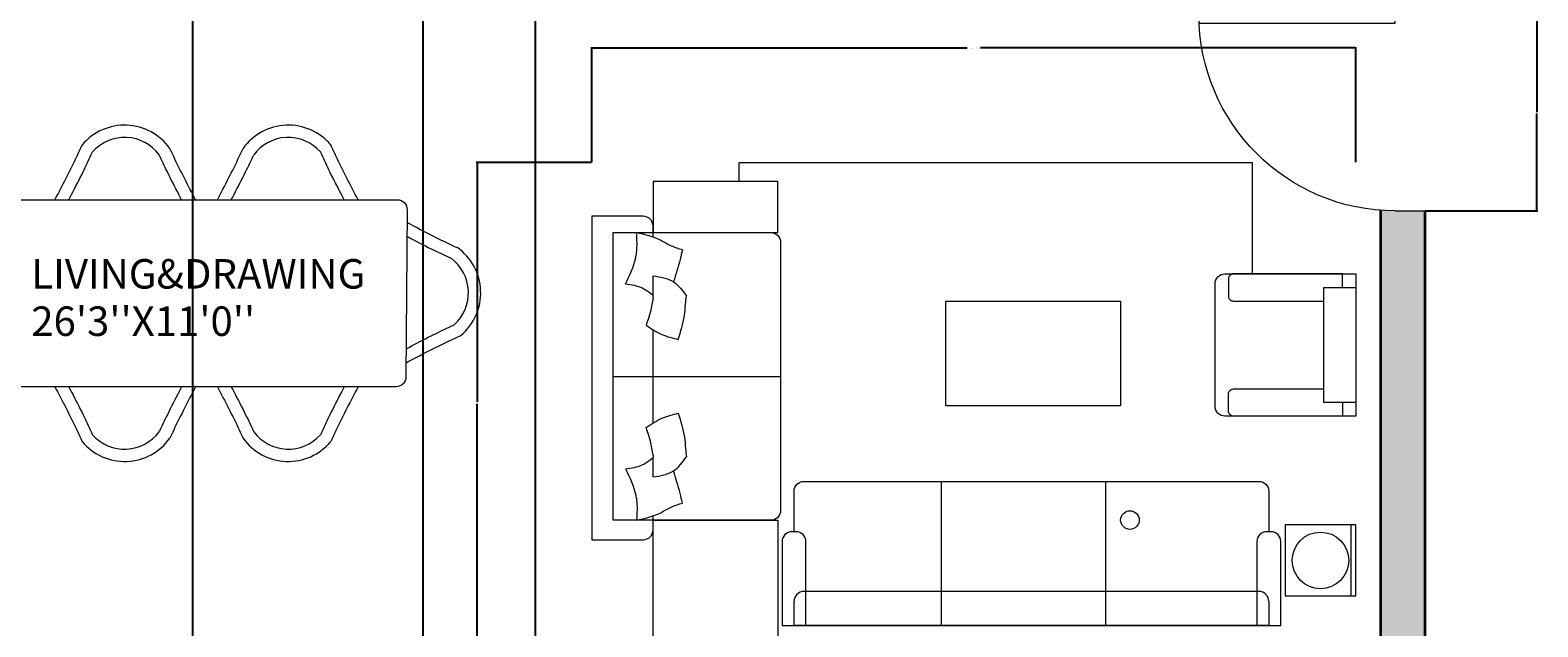
# Model space of a CAD drawing. Units: inches. Extents: x 1789 to 2841, y 3180 to 3702.
# Tile 5 of 14: x 2041 to 2348, y 3388 to 3510. Entities that reach past the tile are written whole.
import ezdxf

# ---------------------------------------------------------------- set-up
doc = ezdxf.new("R2010")
doc.units = ezdxf.units.IN
doc.header["$MEASUREMENT"] = 0
for name, color, linetype, lineweight in [('A-ANNO-DIMS', 2, 'Continuous', 18), ('A-AREA-IDEN', 7, 'Continuous', 18), ('A-WALL', 40, 'Continuous', 35), ('A-WALL-PATT', 252, 'Continuous', 13), ('DORS', 70, 'Continuous', 18), ('FURNITURE', 34, 'Continuous', 18)]:
    doc.layers.add(name, color=color, linetype=linetype, lineweight=lineweight)
doc.styles.get("Standard").update_dxf_attribs({"font": 'arial.ttf'})
doc.dimstyles.get("Standard").update_dxf_attribs({"dimtxt": 0.18, "dimasz": 0.18, "dimexe": 0.18, "dimexo": 0.0625, "dimgap": 0.09, "dimtad": 0, "dimtih": 1, "dimtoh": 1, "dimdec": 0, "dimzin": 0, "dimdsep": 46, "dimlunit": 3, "dimtxsty": 'Standard', "dimcen": 0.09, "dimadec": 0, "dimazin": 0, "dimtfac": 1, "dimtdec": 0, "dimtofl": 0, "dimtmove": 0, "dimatfit": 3, "dimfxl": 1, "dimtolj": 1, "dimtzin": 0, "dimarcsym": 0})

# ---------------------------------------------------------------- blocks, each defined once
blk = doc.blocks.new('*U26')
for p, q in [((0, 0), (0, -6)), ((40, 0), (40, -6))]:
    blk.add_line(p, q)
blk.add_lwpolyline([(0, 0), (0, 40), (1.75, 40), (1.75, 0)], close=True)
blk.add_arc((0, 0), 40, 0, 90)
blk = doc.blocks.new('SOFA')
for p, q in [((2185.57, 3479.13), (2185.57, 3482.99)), ((2185.57, 3482.99), (2290.09, 3482.99)), ((2290.09, 3482.99), (2290.09, 3460.33)), ((2159.93, 3439.46), (2194.03, 3439.46)), ((2226.79, 3388.76), (2226.79, 3418.07)), ((2260.29, 3388.76), (2260.29, 3418.07)), ((2310.14, 3409.22), (2310.14, 3394.77))]:
    blk.add_line(p, q)
for points in [[(2168.05, 3468.75), (2193.44, 3468.75), (2193.44, 3479.13), (2168.05, 3479.13)], [(2227.7, 3454.8), (2263.24, 3454.8), (2263.24, 3433.45), (2227.7, 3433.45)], [(2304.69, 3457.56), (2311.21, 3457.56), (2311.21, 3434.14), (2304.69, 3434.14)], [(2168.05, 3410.16), (2193.44, 3410.16), (2193.44, 3385.14), (2168.05, 3385.14)], [(2296.77, 3394.77), (2311.21, 3394.77), (2311.21, 3409.22), (2296.77, 3409.22)]]:
    blk.add_lwpolyline(points, close=True)
for points in [[(2168.05, 3467.86), (2168.05, 3470.06, 0.414214), (2166.05, 3472.06), (2155.57, 3472.06), (2155.57, 3406.2), (2166.05, 3406.2, 0.414214), (2168.05, 3408.2), (2168.05, 3411.06)], [(2308.49, 3457.56), (2308.49, 3460.33), (2286.26, 3460.33, 0.414214), (2285.26, 3459.33), (2285.26, 3455.79, 0.414214), (2286.26, 3454.79), (2304.69, 3454.79)], [(2308.49, 3434.14), (2308.49, 3431.37), (2286.26, 3431.37, -0.414214), (2285.26, 3432.37), (2285.26, 3435.9, -0.414214), (2286.26, 3436.9), (2304.69, 3436.9)], [(2196.77, 3407.83), (2196.77, 3416.07, -0.414214), (2198.77, 3418.07), (2291.47, 3418.07, -0.414214), (2293.47, 3416.07), (2293.47, 3407.83)], [(2293.47, 3393.66, 0.414214), (2291.47, 3395.66), (2198.77, 3395.66, 0.414214), (2196.77, 3393.66)]]:
    blk.add_lwpolyline(points, format="xyb")
for points in [[(2159.93, 3468.75), (2192.03, 3468.75, -0.414214), (2194.03, 3466.75), (2194.03, 3412.16, -0.414214), (2192.03, 3410.16), (2159.93, 3410.16)], [(2284.53, 3460.33), (2311.21, 3460.33), (2311.21, 3431.37), (2284.53, 3431.37, -0.414214), (2282.53, 3433.37), (2282.53, 3458.33, -0.414214)], [(2197.2, 3407.83), (2196.33, 3407.83, 0.414214), (2194.33, 3405.83), (2194.33, 3388.76), (2199.2, 3388.76), (2199.2, 3405.83, 0.414214)], [(2293.91, 3407.83), (2293.04, 3407.83, 0.414214), (2291.04, 3405.83), (2291.04, 3388.76), (2295.91, 3388.76), (2295.91, 3405.83, 0.414214)]]:
    blk.add_lwpolyline(points, format="xyb", close=True)
for points in [[(2168.05, 3455.52), (2168.05, 3459.94)], [(2168.05, 3429.95), (2168.05, 3448.97)], [(2168.05, 3423.4), (2168.05, 3422.93)], [(2168.05, 3418.98), (2168.05, 3422.93)], [(2293.47, 3393.66), (2293.47, 3388.76), (2196.77, 3388.76), (2196.77, 3393.66)], [(2196.77, 3388.76), (2293.47, 3388.76)]]:
    blk.add_lwpolyline(points)
for centre, radius in [((2265.18, 3410.2), 1.89), ((2303.99, 3401.99), 5.76)]:
    blk.add_circle(centre, radius)
for points, knots in [([(2162.46, 3458.3), (2163.29, 3460.04), (2164.26, 3462.07), (2164.89, 3465.65), (2164.78, 3467.36), (2164.69, 3468.75)], [0, 0, 0, 0, 5.733795, 6.696566, 10.854822, 10.854822, 10.854822, 10.854822]), ([(2164.69, 3468.75), (2166.38, 3468.37), (2168.87, 3467.8), (2171.7, 3465.95), (2173.26, 3465.49), (2174.05, 3465.25)], [0, 0, 0, 0, 5.14676, 7.56322, 10.027291, 10.027291, 10.027291, 10.027291]), ([(2174.05, 3465.25), (2173.89, 3464.58), (2173.37, 3462.38), (2172.69, 3460.22), (2172.22, 3458.71)], [0, 0, 0, 0, 2.055182, 6.796603, 6.796603, 6.796603, 6.796603]), ([(2162.46, 3458.3), (2163.64, 3458.13), (2165.71, 3457.83), (2167.35, 3456.54), (2168.05, 3455.99)], [0, 0, 0, 0, 3.512009, 6.140853, 6.140853, 6.140853, 6.140853]), ([(2168.05, 3459.94), (2169.55, 3459.7), (2172.38, 3459.25), (2174.06, 3456.94), (2174.85, 3455.84)], [0, 0, 0, 0, 4.35123, 8.24052, 8.24052, 8.24052, 8.24052]), ([(2173.18, 3446.97), (2173.68, 3448.57), (2174.42, 3450.93), (2174.65, 3453.95), (2174.79, 3455.29), (2174.85, 3455.84)], [0, 0, 0, 0, 5.016146, 7.373936, 9.056838, 9.056838, 9.056838, 9.056838]), ([(2166.66, 3449.86), (2167.7, 3449.17), (2169.71, 3447.85), (2172.05, 3447.25), (2173.18, 3446.97)], [0, 0, 0, 0, 3.710874, 7.178588, 7.178588, 7.178588, 7.178588]), ([(2166.66, 3429.05), (2167.7, 3429.74), (2169.71, 3431.07), (2172.05, 3431.66), (2173.18, 3431.95)], [0, 0, 0, 0, 3.710874, 7.178588, 7.178588, 7.178588, 7.178588]), ([(2173.18, 3431.95), (2173.68, 3430.35), (2174.42, 3427.99), (2174.65, 3424.97), (2174.79, 3423.63), (2174.85, 3423.07)], [0, 0, 0, 0, 5.016146, 7.373936, 9.056838, 9.056838, 9.056838, 9.056838]), ([(2162.46, 3420.62), (2163.64, 3420.79), (2165.71, 3421.09), (2167.35, 3422.37), (2168.05, 3422.93)], [0, 0, 0, 0, 3.512009, 6.140853, 6.140853, 6.140853, 6.140853]), ([(2168.05, 3418.98), (2169.55, 3419.22), (2172.38, 3419.66), (2174.06, 3421.98), (2174.85, 3423.07)], [0, 0, 0, 0, 4.35123, 8.24052, 8.24052, 8.24052, 8.24052]), ([(2162.46, 3420.62), (2163.29, 3418.88), (2164.26, 3416.85), (2164.89, 3413.27), (2164.78, 3411.56), (2164.69, 3410.16)], [0, 0, 0, 0, 5.733795, 6.696566, 10.854822, 10.854822, 10.854822, 10.854822]), ([(2174.05, 3413.67), (2173.89, 3414.33), (2173.37, 3416.54), (2172.69, 3418.7), (2172.22, 3420.21)], [0, 0, 0, 0, 2.055182, 6.796603, 6.796603, 6.796603, 6.796603]), ([(2164.69, 3410.16), (2166.38, 3410.55), (2168.87, 3411.12), (2171.7, 3412.96), (2173.26, 3413.43), (2174.05, 3413.67)], [0, 0, 0, 0, 5.14676, 7.56322, 10.027291, 10.027291, 10.027291, 10.027291])]:
    blk.add_open_spline(points, degree=3, knots=knots)
for points in [[(2168.05, 3455.52), (2167.85, 3453.6), (2167.25, 3451.73), (2166.66, 3449.86)], [(2168.05, 3423.4), (2167.85, 3425.31), (2167.25, 3427.18), (2166.66, 3429.05)]]:
    blk.add_open_spline(points, degree=3)
blk = doc.blocks.new('DINI')
blk.add_lwpolyline([(2038.22, 3475.42), (2115.97, 3475.42, -0.414214), (2117.97, 3473.42), (2117.72, 3439.35, -0.414214), (2115.72, 3437.35), (2037.97, 3437.35, -0.414214), (2035.97, 3439.35), (2036.22, 3473.42, -0.414214)], format="xyb", close=True)
for centre, radius, start, end in [((2060.43, 3479.31), 11.31, 35.4017, 140.0736), ((2093.76, 3479.31), 11.31, 39.9264, 144.5983), ((2060.43, 3479.31), 8.8, 36.8657, 137.9611), ((2093.76, 3479.31), 8.8, 42.0389, 143.1343), ((2032.05, 3456.46), 11.31, 125.4017, 230.0736), ((2121.64, 3456.46), 11.31, 309.9264, 54.5983), ((2032.05, 3456.46), 8.8, 126.8657, 227.9611), ((2121.64, 3456.46), 8.8, 312.0389, 53.1343), ((2060.43, 3433.45), 8.8, 222.0389, 323.1343), ((2093.76, 3433.45), 8.8, 216.8657, 317.9611), ((2060.43, 3433.45), 11.31, 219.9264, 324.5983), ((2093.76, 3433.45), 11.31, 215.4017, 320.0736)]:
    blk.add_arc(centre, radius, start, end)
for points, knots in [([(2046.22, 3475.42), (2047.75, 3478.33), (2049.68, 3482.01), (2051.4, 3485.79), (2051.76, 3486.58)], [0, 0, 0, 0, 7.856931, 9.915256, 9.915256, 9.915256, 9.915256]), ([(2074.88, 3475.42), (2073.35, 3478.33), (2071.54, 3481.78), (2069.91, 3485.32), (2069.66, 3485.87)], [0, 0, 0, 0, 7.856931, 9.297576, 9.297576, 9.297576, 9.297576]), ([(2079.31, 3475.42), (2080.85, 3478.33), (2082.66, 3481.78), (2084.29, 3485.32), (2084.54, 3485.87)], [0, 0, 0, 0, 7.856931, 9.297576, 9.297576, 9.297576, 9.297576]), ([(2107.98, 3475.42), (2106.45, 3478.33), (2104.51, 3482.01), (2102.79, 3485.79), (2102.44, 3486.58)], [0, 0, 0, 0, 7.856931, 9.915256, 9.915256, 9.915256, 9.915256]), ([(2049.05, 3475.42), (2049.25, 3475.79), (2049.44, 3476.15), (2050.42, 3478.03), (2051.21, 3479.56), (2052.54, 3482.27), (2053.1, 3483.45), (2053.72, 3484.82), (2053.81, 3485.01), (2053.9, 3485.21)], [1.048693, 1.048693, 1.048693, 1.048693, 2.029233, 2.029233, 6.0877, 6.0877, 9.118148, 9.118148, 9.624349, 9.624349, 9.624349, 9.624349]), ([(2072.04, 3475.42), (2071.85, 3475.78), (2071.66, 3476.15), (2070.68, 3478.03), (2069.89, 3479.55), (2068.56, 3482.26), (2068.01, 3483.43), (2067.48, 3484.59)], [1.048889, 1.048889, 1.048889, 1.048889, 2.02655, 2.02655, 6.079649, 6.079649, 9.095857, 9.095857, 9.095857, 9.095857]), ([(2082.15, 3475.42), (2082.34, 3475.78), (2082.53, 3476.15), (2083.51, 3478.03), (2084.3, 3479.55), (2085.63, 3482.26), (2086.19, 3483.43), (2086.72, 3484.59)], [1.048889, 1.048889, 1.048889, 1.048889, 2.02655, 2.02655, 6.079649, 6.079649, 9.095857, 9.095857, 9.095857, 9.095857]), ([(2105.14, 3475.42), (2104.95, 3475.79), (2104.76, 3476.15), (2103.78, 3478.03), (2102.99, 3479.56), (2101.65, 3482.27), (2101.1, 3483.45), (2100.47, 3484.82), (2100.38, 3485.01), (2100.3, 3485.21)], [1.048693, 1.048693, 1.048693, 1.048693, 2.029233, 2.029233, 6.0877, 6.0877, 9.118148, 9.118148, 9.624349, 9.624349, 9.624349, 9.624349]), ([(2036.2, 3471.04), (2036.05, 3470.96), (2035.89, 3470.88), (2035.74, 3470.8), (2035.74, 3470.8), (2035.74, 3470.8), (2035.74, 3470.8), (2032.89, 3469.3), (2029.51, 3467.53), (2026.05, 3465.93), (2025.5, 3465.68)], [-0.229823, -0.229823, -0.229823, -0.229823, 0.189373, 0.189373, 0.189373, 0.189712, 0.189712, 0.189712, 7.856931, 9.297576, 9.297576, 9.297576, 9.297576]), ([(2117.95, 3470.8), (2120.8, 3469.3), (2124.18, 3467.53), (2127.64, 3465.93), (2128.19, 3465.68)], [0.189712, 0.189712, 0.189712, 0.189712, 7.856931, 9.297576, 9.297576, 9.297576, 9.297576]), ([(2036.18, 3468.19), (2036.04, 3468.12), (2035.9, 3468.04), (2035.76, 3467.97), (2035.76, 3467.97), (2035.76, 3467.97), (2035.76, 3467.97), (2035.46, 3467.81), (2035.16, 3467.65), (2033.34, 3466.71), (2031.81, 3465.92), (2029.11, 3464.59), (2027.94, 3464.04), (2026.77, 3463.5)], [0.838882, 0.838882, 0.838882, 0.838882, 1.215073, 1.215073, 1.215073, 1.219193, 1.219193, 1.219193, 2.02655, 2.02655, 6.079649, 6.079649, 9.095857, 9.095857, 9.095857, 9.095857]), ([(2117.93, 3467.97), (2118.23, 3467.81), (2118.53, 3467.65), (2120.35, 3466.71), (2121.88, 3465.92), (2124.58, 3464.59), (2125.75, 3464.04), (2126.92, 3463.5)], [1.219193, 1.219193, 1.219193, 1.219193, 2.02655, 2.02655, 6.079649, 6.079649, 9.095857, 9.095857, 9.095857, 9.095857]), ([(2035.95, 3445.08), (2035.58, 3445.27), (2035.22, 3445.46), (2033.34, 3446.45), (2031.81, 3447.23), (2029.1, 3448.57), (2027.92, 3449.12), (2026.55, 3449.75), (2026.36, 3449.84), (2026.16, 3449.93)], [1.048693, 1.048693, 1.048693, 1.048693, 2.029233, 2.029233, 6.0877, 6.0877, 9.118148, 9.118148, 9.624349, 9.624349, 9.624349, 9.624349]), ([(2117.74, 3445.08), (2118.11, 3445.27), (2118.47, 3445.46), (2120.35, 3446.45), (2121.88, 3447.23), (2124.59, 3448.57), (2125.77, 3449.12), (2127.14, 3449.75), (2127.33, 3449.84), (2127.53, 3449.93)], [1.048693, 1.048693, 1.048693, 1.048693, 2.029233, 2.029233, 6.0877, 6.0877, 9.118148, 9.118148, 9.624349, 9.624349, 9.624349, 9.624349]), ([(2035.95, 3442.24), (2033.03, 3443.77), (2029.36, 3445.71), (2025.58, 3447.43), (2024.79, 3447.79)], [0, 0, 0, 0, 7.856931, 9.915256, 9.915256, 9.915256, 9.915256]), ([(2117.74, 3442.24), (2120.66, 3443.77), (2124.33, 3445.71), (2128.11, 3447.43), (2128.9, 3447.79)], [0, 0, 0, 0, 7.856931, 9.915256, 9.915256, 9.915256, 9.915256]), ([(2046.22, 3437.35), (2047.75, 3434.43), (2049.68, 3430.75), (2051.4, 3426.98), (2051.76, 3426.19)], [0, 0, 0, 0, 7.856931, 9.915256, 9.915256, 9.915256, 9.915256]), ([(2049.05, 3437.35), (2049.25, 3436.98), (2049.44, 3436.62), (2050.42, 3434.73), (2051.21, 3433.2), (2052.54, 3430.5), (2053.1, 3429.32), (2053.72, 3427.95), (2053.81, 3427.75), (2053.9, 3427.56)], [1.048693, 1.048693, 1.048693, 1.048693, 2.029233, 2.029233, 6.0877, 6.0877, 9.118148, 9.118148, 9.624349, 9.624349, 9.624349, 9.624349]), ([(2072.04, 3437.35), (2071.85, 3436.98), (2071.66, 3436.62), (2070.68, 3434.74), (2069.89, 3433.21), (2068.56, 3430.51), (2068.01, 3429.34), (2067.48, 3428.17)], [1.048889, 1.048889, 1.048889, 1.048889, 2.02655, 2.02655, 6.079649, 6.079649, 9.095857, 9.095857, 9.095857, 9.095857]), ([(2074.88, 3437.35), (2073.35, 3434.43), (2071.54, 3430.98), (2069.91, 3427.45), (2069.66, 3426.9)], [0, 0, 0, 0, 7.856931, 9.297576, 9.297576, 9.297576, 9.297576]), ([(2079.31, 3437.35), (2080.85, 3434.43), (2082.66, 3430.98), (2084.29, 3427.45), (2084.54, 3426.9)], [0, 0, 0, 0, 7.856931, 9.297576, 9.297576, 9.297576, 9.297576]), ([(2082.15, 3437.35), (2082.34, 3436.98), (2082.53, 3436.62), (2083.51, 3434.74), (2084.3, 3433.21), (2085.63, 3430.51), (2086.19, 3429.34), (2086.72, 3428.17)], [1.048889, 1.048889, 1.048889, 1.048889, 2.02655, 2.02655, 6.079649, 6.079649, 9.095857, 9.095857, 9.095857, 9.095857]), ([(2105.14, 3437.35), (2104.95, 3436.98), (2104.76, 3436.62), (2103.78, 3434.73), (2102.99, 3433.2), (2101.65, 3430.5), (2101.1, 3429.32), (2100.47, 3427.95), (2100.38, 3427.75), (2100.3, 3427.56)], [1.048693, 1.048693, 1.048693, 1.048693, 2.029233, 2.029233, 6.0877, 6.0877, 9.118148, 9.118148, 9.624349, 9.624349, 9.624349, 9.624349]), ([(2107.98, 3437.35), (2106.45, 3434.43), (2104.51, 3430.75), (2102.79, 3426.98), (2102.44, 3426.19)], [0, 0, 0, 0, 7.856931, 9.915256, 9.915256, 9.915256, 9.915256])]:
    blk.add_open_spline(points, degree=3, knots=knots)
blk = doc.blocks.new('*D67')
at = {"layer": 'A-ANNO-DIMS', "color": 0, "lineweight": -2, "transparency": 16777216}
for p, q in [((2155.57, 3483.05), (2155.57, 3506.51)), ((2155.75, 3506.33), (2232.02, 3506.33)), ((2311.03, 3506.33), (2234.76, 3506.33)), ((2311.21, 3483.05), (2311.21, 3506.51))]:
    blk.add_line(p, q, dxfattribs=at)
at = {"layer": 'A-ANNO-DIMS', "color": 0, "transparency": 16777216}
for points in [[(2155.75, 3506.36), (2155.75, 3506.3), (2155.57, 3506.33)], [(2311.03, 3506.36), (2311.03, 3506.3), (2311.21, 3506.33)]]:
    blk.add_solid(points, dxfattribs=at)
at = {"layer": 'Defpoints', "color": 0, "transparency": 16777216}
for p in [(2311.21, 3506.33), (2155.57, 3482.99), (2311.21, 3482.99)]:
    blk.add_point(p, dxfattribs=at)
at = {"layer": 'A-ANNO-DIMS', "color": 0, "transparency": 16777216, "insert": (2233.39, 3506.33), "char_height": 0.18, "attachment_point": 5}
blk.add_mtext('\\A1;SEATING GROUP 156', dxfattribs=at)
blk = doc.blocks.new('*D68')
at = {"layer": 'A-ANNO-DIMS', "color": 0, "lineweight": -2, "transparency": 16777216}
for p, q in [((2155.51, 3482.99), (2132.05, 3482.99)), ((2132.23, 3482.81), (2132.23, 3434.25)), ((2132.23, 3385.32), (2132.23, 3433.88)), ((2155.51, 3385.14), (2132.05, 3385.14))]:
    blk.add_line(p, q, dxfattribs=at)
at = {"layer": 'A-ANNO-DIMS', "color": 0, "transparency": 16777216}
for points in [[(2132.2, 3482.81), (2132.26, 3482.81), (2132.23, 3482.99)], [(2132.2, 3385.32), (2132.26, 3385.32), (2132.23, 3385.14)]]:
    blk.add_solid(points, dxfattribs=at)
at = {"layer": 'Defpoints', "color": 0, "transparency": 16777216}
for p in [(2132.23, 3482.99), (2155.57, 3482.99), (2155.57, 3385.14)]:
    blk.add_point(p, dxfattribs=at)
at = {"layer": 'A-ANNO-DIMS', "color": 0, "transparency": 16777216, "insert": (2132.23, 3434.07), "char_height": 0.18, "attachment_point": 5}
blk.add_mtext('\\A1;98', dxfattribs=at)
blk = doc.blocks.new('*D88')
at = {"layer": 'A-ANNO-DIMS', "color": 0, "lineweight": -2, "transparency": 16777216}
for p, q in [((2325.3, 3513.16), (2348.26, 3513.16)), ((2348.08, 3512.98), (2348.08, 3493.34)), ((2348.08, 3473.34), (2348.08, 3492.98)), ((2325.3, 3473.16), (2348.26, 3473.16))]:
    blk.add_line(p, q, dxfattribs=at)
at = {"layer": 'A-ANNO-DIMS', "color": 0, "transparency": 16777216}
for points in [[(2348.05, 3512.98), (2348.11, 3512.98), (2348.08, 3513.16)], [(2348.05, 3473.34), (2348.11, 3473.34), (2348.08, 3473.16)]]:
    blk.add_solid(points, dxfattribs=at)
at = {"layer": 'Defpoints', "color": 0, "transparency": 16777216}
for p in [(2325.23, 3513.16), (2325.23, 3473.16), (2348.08, 3473.16)]:
    blk.add_point(p, dxfattribs=at)
at = {"layer": 'A-ANNO-DIMS', "color": 0, "transparency": 16777216, "insert": (2348.08, 3493.16), "char_height": 0.18, "attachment_point": 5}
blk.add_mtext('\\A1;40', dxfattribs=at)
blk = doc.blocks.new('*D90')
at = {"layer": 'A-ANNO-DIMS', "color": 0, "lineweight": -2, "transparency": 16777216}
for p, q in [((2038.23, 3517.1), (2038.23, 3180.13)), ((2074.23, 3517.1), (2074.23, 3180.13)), ((2038.41, 3180.31), (2056.01, 3180.31)), ((2074.05, 3180.31), (2056.45, 3180.31))]:
    blk.add_line(p, q, dxfattribs=at)
at = {"layer": 'A-ANNO-DIMS', "color": 0, "transparency": 16777216}
for points in [[(2038.41, 3180.34), (2038.41, 3180.28), (2038.23, 3180.31)], [(2074.05, 3180.34), (2074.05, 3180.28), (2074.23, 3180.31)]]:
    blk.add_solid(points, dxfattribs=at)
at = {"layer": 'Defpoints', "color": 0, "transparency": 16777216}
for p in [(2038.23, 3517.16), (2074.23, 3517.16), (2074.23, 3180.31)]:
    blk.add_point(p, dxfattribs=at)
at = {"layer": 'A-ANNO-DIMS', "color": 0, "transparency": 16777216, "insert": (2056.23, 3180.31), "char_height": 0.18, "attachment_point": 5}
blk.add_mtext('\\A1;36', dxfattribs=at)
blk = doc.blocks.new('*D91')
at = {"layer": 'A-ANNO-DIMS', "color": 0, "lineweight": -2, "transparency": 16777216}
for p, q in [((2121.23, 3385.22), (2121.23, 3678.19)), ((2121.41, 3678.01), (2132.21, 3678.01)), ((2143.93, 3678.01), (2133.14, 3678.01)), ((2144.11, 3385.22), (2144.11, 3678.19))]:
    blk.add_line(p, q, dxfattribs=at)
at = {"layer": 'A-ANNO-DIMS', "color": 0, "transparency": 16777216}
for points in [[(2121.41, 3678.04), (2121.41, 3677.98), (2121.23, 3678.01)], [(2143.93, 3678.04), (2143.93, 3677.98), (2144.11, 3678.01)]]:
    blk.add_solid(points, dxfattribs=at)
at = {"layer": 'Defpoints', "color": 0, "transparency": 16777216}
for p in [(2144.11, 3678.01), (2121.23, 3385.16), (2144.11, 3385.16)]:
    blk.add_point(p, dxfattribs=at)
at = {"layer": 'A-ANNO-DIMS', "color": 0, "transparency": 16777216, "insert": (2132.67, 3678.01), "char_height": 0.18, "attachment_point": 5}
blk.add_mtext('\\A1;22.875', dxfattribs=at)
blk = doc.blocks.new('*D116')
at = {"layer": 'A-ANNO-DIMS', "color": 0, "lineweight": -2, "transparency": 16777216}
for p, q in [((1789.65, 3701.85), (1789.83, 3701.85)), ((1789.83, 3701.85), (1945.65, 3528.3)), ((2205.56, 3238.68), (2205.74, 3238.68)), ((2205.65, 3238.59), (2205.65, 3238.77))]:
    blk.add_line(p, q, dxfattribs=at)
at = {"layer": 'A-ANNO-DIMS', "color": 0, "transparency": 16777216}
blk.add_solid([(1945.67, 3528.32), (1945.62, 3528.28), (1945.77, 3528.16)], dxfattribs=at)
at = {"layer": 'Defpoints', "color": 0, "transparency": 16777216}
for p in [(1945.77, 3528.16), (2205.65, 3238.68)]:
    blk.add_point(p, dxfattribs=at)
at = {"layer": 'A-ANNO-DIMS', "color": 0, "transparency": 16777216, "insert": (1789.28, 3701.85), "char_height": 0.18, "attachment_point": 5}
blk.add_mtext('\\A1;R389', dxfattribs=at)

msp = doc.modelspace()

# ---------------------------------------------------------------- hatches: boundary and pattern name
at = {"layer": 'A-WALL-PATT'}
h = msp.add_hatch(color=256, dxfattribs=at)
h.dxf.hatch_style = 1
h.paths.add_polyline_path([(2316.2333, 3385.1608), (2193.4449, 3385.1608), (2193.4449, 3385.1441), (2181.2333, 3385.1441), (2181.2333, 3376.1608), (2316.2333, 3376.1608), (2316.2333, 3279.1608), (2244.9532, 3279.1608), (2244.9532, 3272.1608), (2316.2333, 3272.1608), (2316.2333, 3212.1608), (2273.8514, 3212.1608), (2273.8514, 3203.1608), (2325.2333, 3203.1608), (2325.2333, 3473.1608), (2319.2333, 3473.1608, -0.01876983), (2316.2333, 3473.2734)])

# ---------------------------------------------------------------- linework, layer by layer
at = {"layer": 'A-WALL'}
for p, q in [((2316.2333, 3473.2734), (2316.2333, 3385.1608)), ((2325.2333, 3473.1608), (2325.2333, 3203.1608))]:
    msp.add_line(p, q, dxfattribs=at)

# ---------------------------------------------------------------- block references
at = {"layer": 'DORS', "xscale": -1, "rotation": 90}
msp.add_blockref('*U26', (2319.2333, 3513.1608), dxfattribs=at)
at = {"layer": 'FURNITURE'}
for name in ['DINI', 'SOFA']:
    msp.add_blockref(name, (0, 0), dxfattribs=at)

# ---------------------------------------------------------------- texts
at = {"layer": 'A-ANNO-DIMS'}
msp.add_text("26'3''X11'0''", height=6, dxfattribs=at).set_placement((2041.4097, 3447.6999))
at = {"layer": 'A-AREA-IDEN'}
msp.add_text('LIVING&DRAWING', height=6, dxfattribs=at).set_placement((2041.4097, 3457.3383))

# ---------------------------------------------------------------- dimensions: what is measured, and where the dimension line sits
at = {"layer": 'A-ANNO-DIMS'}
dim = msp.add_radius_dim(center=(2205.6545, 3238.6823), mpoint=(1945.766, 3528.162), dimstyle='Standard', override={"dimdec": 0, "dimlfac": 1, "dimrnd": 0, "dimzin": 0, "dimdsep": 46, "dimlunit": 2}, dxfattribs=at)
dim.commit()
dim.dimension.update_dxf_attribs({"geometry": '*D116', "text_midpoint": (1789.2778, 3701.8498), "dimtype": 164})
for base, p1, p2, override, picture, middle in [((2144.1086, 3678.0108), (2121.2333, 3385.1608), (2144.1086, 3385.1608), {"dimdec": 3, "dimlfac": 1, "dimrnd": 0, "dimzin": 0, "dimdsep": 46, "dimlunit": 2}, '*D91', (2132.671, 3678.0108)), ((2074.2333, 3180.3108), (2038.2333, 3517.1608), (2074.2333, 3517.1608), {"dimdec": 0, "dimlfac": 1, "dimrnd": 0, "dimzin": 0, "dimdsep": 46, "dimlunit": 2}, '*D90', (2056.2333, 3180.3108))]:
    dim = msp.add_linear_dim(base=base, p1=p1, p2=p2, dimstyle='Standard', override=override, dxfattribs=at)
    dim.commit()
    dim.dimension.update_dxf_attribs({"geometry": picture, "text_midpoint": middle})
for base, p1, p2, picture, middle in [((2348.0833, 3473.1608), (2325.2333, 3513.1608), (2325.2333, 3473.1608), '*D88', (2348.0833, 3493.1608)), ((2132.226, 3482.9891), (2155.5718, 3385.1441), (2155.5718, 3482.9891), '*D68', (2132.226, 3434.0666))]:
    dim = msp.add_linear_dim(base=base, p1=p1, p2=p2, angle=90, dimstyle='Standard', override={"dimdec": 0, "dimlfac": 1, "dimrnd": 0, "dimzin": 0, "dimdsep": 46, "dimlunit": 2}, dxfattribs=at)
    dim.commit()
    dim.dimension.update_dxf_attribs({"geometry": picture, "text_midpoint": middle})
dim = msp.add_linear_dim(base=(2311.2105, 3506.335), p1=(2155.5718, 3482.9891), p2=(2311.2105, 3482.9891), text='SEATING GROUP <>', dimstyle='Standard', override={"dimdec": 0, "dimlfac": 1, "dimrnd": 0, "dimzin": 0, "dimdsep": 46, "dimlunit": 2}, dxfattribs=at)
dim.commit()
dim.dimension.update_dxf_attribs({"geometry": '*D67', "text_midpoint": (2233.3911, 3506.335)})

doc.saveas('drawing.dxf')
